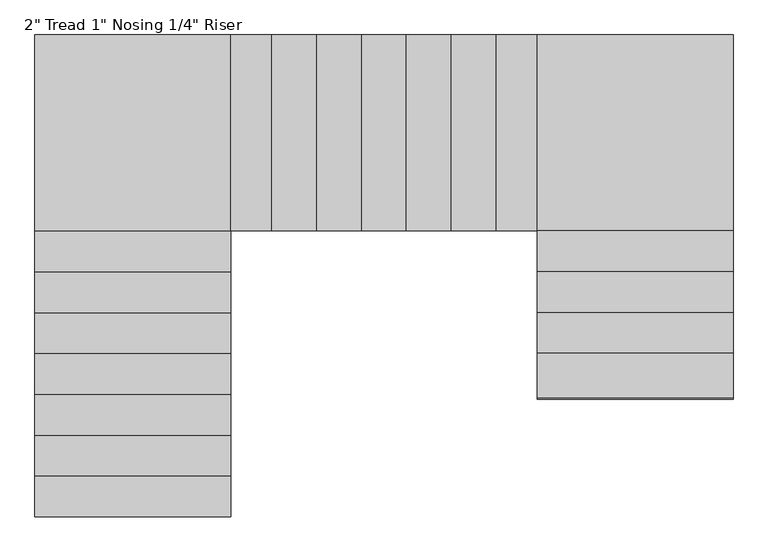
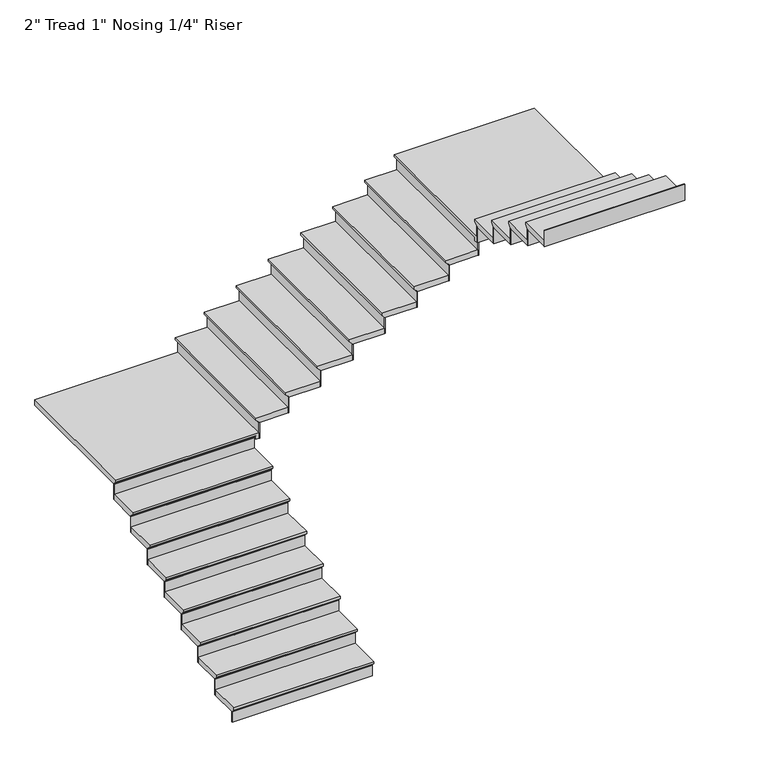
"""IFC4 building model written with IfcOpenShell, lengths in millimetres: stair flight geometry."""

from ifc_helpers import new_model, si_unit, origin, place, context, project, spatial, faceted_brep, source, transform, mapped, element, save


def stair_flight_02d0fc9c(model_context):
    return source(origin(), model_context, "Body", "Brep", [
        faceted_brep([(-39503.1146233, 12686.9618061, 6374.4928571), (-39503.1146233, 12686.9618061, 6393.5428571), (-40722.3146233, 12686.9618061, 6393.5428571), (-40722.3146233, 12686.9618061, 6374.4928571), (-39503.1146233, 12712.3618061, 6349.0928571), (-40722.3146233, 12712.3618061, 6349.0928571), (-39503.1146233, 12966.3618061, 6393.5428571), (-40722.3146233, 12966.3618061, 6393.5428571), (-40722.3146233, 12712.3618061, 6342.7428571), (-40722.3146233, 12966.3618061, 6342.7428571), (-39503.1146233, 12966.3618061, 6342.7428571), (-39503.1146233, 12712.3618061, 6342.7428571)], [[[0, 1, 2, 3]], [[4, 0, 3, 5]], [[2, 1, 6, 7]], [[8, 9, 10, 11]], [[2, 7, 9, 8, 5, 3]], [[8, 11, 4, 5]], [[6, 1, 0, 4, 11, 10]], [[7, 6, 10, 9]]]),
        faceted_brep([(-39503.1146233, 12712.3618061, 6342.7428571), (-39503.1146233, 12712.3618061, 6248.4), (-39503.1146233, 12718.7118061, 6248.4), (-39503.1146233, 12718.7118061, 6342.7428571), (-40722.3146233, 12712.3618061, 6342.7428571), (-40722.3146233, 12718.7118061, 6342.7428571), (-40722.3146233, 12718.7118061, 6248.4), (-40722.3146233, 12712.3618061, 6248.4)], [[[0, 1, 2, 3]], [[4, 5, 6, 7]], [[1, 0, 4, 7]], [[2, 1, 7, 6]], [[3, 2, 6, 5]], [[0, 3, 5, 4]]]),
        faceted_brep([(-39503.1146233, 12966.3618061, 6487.8857143), (-39503.1146233, 12966.3618061, 6342.7428571), (-39503.1146233, 12972.7118061, 6342.7428571), (-39503.1146233, 12972.7118061, 6487.8857143), (-40722.3146233, 12966.3618061, 6487.8857143), (-40722.3146233, 12972.7118061, 6487.8857143), (-40722.3146233, 12972.7118061, 6342.7428571), (-40722.3146233, 12966.3618061, 6342.7428571)], [[[0, 1, 2, 3]], [[4, 5, 6, 7]], [[1, 0, 4, 7]], [[2, 1, 7, 6]], [[3, 2, 6, 5]], [[0, 3, 5, 4]]]),
        faceted_brep([(-40722.3146233, 12940.9618061, 6538.6857143), (-39503.1146233, 12940.9618061, 6538.6857143), (-39503.1146233, 13220.3618061, 6538.6857143), (-40722.3146233, 13220.3618061, 6538.6857143), (-40722.3146233, 12966.3618061, 6487.8857143), (-40722.3146233, 13220.3618061, 6487.8857143), (-39503.1146233, 13220.3618061, 6487.8857143), (-39503.1146233, 12966.3618061, 6487.8857143), (-40722.3146233, 12966.3618061, 6494.2357143), (-40722.3146233, 12940.9618061, 6519.6357143), (-39503.1146233, 12966.3618061, 6494.2357143), (-39503.1146233, 12940.9618061, 6519.6357143)], [[[0, 1, 2, 3]], [[4, 5, 6, 7]], [[0, 3, 5, 4, 8, 9]], [[4, 7, 10, 8]], [[2, 1, 11, 10, 7, 6]], [[3, 2, 6, 5]], [[11, 1, 0, 9]], [[10, 11, 9, 8]]]),
        faceted_brep([(-39503.1146233, 13220.3618061, 6633.0285714), (-39503.1146233, 13220.3618061, 6487.8857143), (-39503.1146233, 13226.7118061, 6487.8857143), (-39503.1146233, 13226.7118061, 6633.0285714), (-40722.3146233, 13220.3618061, 6633.0285714), (-40722.3146233, 13226.7118061, 6633.0285714), (-40722.3146233, 13226.7118061, 6487.8857143), (-40722.3146233, 13220.3618061, 6487.8857143)], [[[0, 1, 2, 3]], [[4, 5, 6, 7]], [[1, 0, 4, 7]], [[2, 1, 7, 6]], [[3, 2, 6, 5]], [[0, 3, 5, 4]]]),
        faceted_brep([(-40722.3146233, 13194.9618061, 6683.8285714), (-39503.1146233, 13194.9618061, 6683.8285714), (-39503.1146233, 13474.3618061, 6683.8285714), (-40722.3146233, 13474.3618061, 6683.8285714), (-40722.3146233, 13220.3618061, 6633.0285714), (-40722.3146233, 13474.3618061, 6633.0285714), (-39503.1146233, 13474.3618061, 6633.0285714), (-39503.1146233, 13220.3618061, 6633.0285714), (-40722.3146233, 13220.3618061, 6639.3785714), (-40722.3146233, 13194.9618061, 6664.7785714), (-39503.1146233, 13220.3618061, 6639.3785714), (-39503.1146233, 13194.9618061, 6664.7785714)], [[[0, 1, 2, 3]], [[4, 5, 6, 7]], [[0, 3, 5, 4, 8, 9]], [[4, 7, 10, 8]], [[2, 1, 11, 10, 7, 6]], [[3, 2, 6, 5]], [[11, 1, 0, 9]], [[10, 11, 9, 8]]]),
        faceted_brep([(-39503.1146233, 13474.3618061, 6778.1714286), (-39503.1146233, 13474.3618061, 6633.0285714), (-39503.1146233, 13480.7118061, 6633.0285714), (-39503.1146233, 13480.7118061, 6778.1714286), (-40722.3146233, 13474.3618061, 6778.1714286), (-40722.3146233, 13480.7118061, 6778.1714286), (-40722.3146233, 13480.7118061, 6633.0285714), (-40722.3146233, 13474.3618061, 6633.0285714)], [[[0, 1, 2, 3]], [[4, 5, 6, 7]], [[1, 0, 4, 7]], [[2, 1, 7, 6]], [[3, 2, 6, 5]], [[0, 3, 5, 4]]]),
        faceted_brep([(-40722.3146233, 13448.9618061, 6828.9714286), (-39503.1146233, 13448.9618061, 6828.9714286), (-39503.1146233, 13728.3618061, 6828.9714286), (-40722.3146233, 13728.3618061, 6828.9714286), (-40722.3146233, 13474.3618061, 6778.1714286), (-40722.3146233, 13728.3618061, 6778.1714286), (-39503.1146233, 13728.3618061, 6778.1714286), (-39503.1146233, 13474.3618061, 6778.1714286), (-40722.3146233, 13474.3618061, 6784.5214286), (-40722.3146233, 13448.9618061, 6809.9214286), (-39503.1146233, 13474.3618061, 6784.5214286), (-39503.1146233, 13448.9618061, 6809.9214286)], [[[0, 1, 2, 3]], [[4, 5, 6, 7]], [[0, 3, 5, 4, 8, 9]], [[4, 7, 10, 8]], [[2, 1, 11, 10, 7, 6]], [[3, 2, 6, 5]], [[11, 1, 0, 9]], [[10, 11, 9, 8]]]),
        faceted_brep([(-39503.1146233, 13728.3618061, 6923.3142857), (-39503.1146233, 13728.3618061, 6778.1714286), (-39503.1146233, 13734.7118061, 6778.1714286), (-39503.1146233, 13734.7118061, 6923.3142857), (-40722.3146233, 13728.3618061, 6923.3142857), (-40722.3146233, 13734.7118061, 6923.3142857), (-40722.3146233, 13734.7118061, 6778.1714286), (-40722.3146233, 13728.3618061, 6778.1714286)], [[[0, 1, 2, 3]], [[4, 5, 6, 7]], [[1, 0, 4, 7]], [[2, 1, 7, 6]], [[3, 2, 6, 5]], [[0, 3, 5, 4]]]),
        faceted_brep([(-40722.3146233, 13702.9618061, 6974.1142857), (-39503.1146233, 13702.9618061, 6974.1142857), (-39503.1146233, 13982.3618061, 6974.1142857), (-40722.3146233, 13982.3618061, 6974.1142857), (-40722.3146233, 13728.3618061, 6923.3142857), (-40722.3146233, 13982.3618061, 6923.3142857), (-39503.1146233, 13982.3618061, 6923.3142857), (-39503.1146233, 13728.3618061, 6923.3142857), (-40722.3146233, 13728.3618061, 6929.6642857), (-40722.3146233, 13702.9618061, 6955.0642857), (-39503.1146233, 13728.3618061, 6929.6642857), (-39503.1146233, 13702.9618061, 6955.0642857)], [[[0, 1, 2, 3]], [[4, 5, 6, 7]], [[0, 3, 5, 4, 8, 9]], [[4, 7, 10, 8]], [[2, 1, 11, 10, 7, 6]], [[3, 2, 6, 5]], [[11, 1, 0, 9]], [[10, 11, 9, 8]]]),
        faceted_brep([(-39503.1146233, 13982.3618061, 7068.4571429), (-39503.1146233, 13982.3618061, 6923.3142857), (-39503.1146233, 13988.7118061, 6923.3142857), (-39503.1146233, 13988.7118061, 7068.4571429), (-40722.3146233, 13982.3618061, 7068.4571429), (-40722.3146233, 13988.7118061, 7068.4571429), (-40722.3146233, 13988.7118061, 6923.3142857), (-40722.3146233, 13982.3618061, 6923.3142857)], [[[0, 1, 2, 3]], [[4, 5, 6, 7]], [[1, 0, 4, 7]], [[2, 1, 7, 6]], [[3, 2, 6, 5]], [[0, 3, 5, 4]]]),
        faceted_brep([(-40722.3146233, 13956.9618061, 7119.2571429), (-39503.1146233, 13956.9618061, 7119.2571429), (-39503.1146233, 14236.3618061, 7119.2571429), (-40722.3146233, 14236.3618061, 7119.2571429), (-40722.3146233, 13982.3618061, 7068.4571429), (-40722.3146233, 14236.3618061, 7068.4571429), (-39503.1146233, 14236.3618061, 7068.4571429), (-39503.1146233, 13982.3618061, 7068.4571429), (-40722.3146233, 13982.3618061, 7074.8071429), (-40722.3146233, 13956.9618061, 7100.2071429), (-39503.1146233, 13982.3618061, 7074.8071429), (-39503.1146233, 13956.9618061, 7100.2071429)], [[[0, 1, 2, 3]], [[4, 5, 6, 7]], [[0, 3, 5, 4, 8, 9]], [[4, 7, 10, 8]], [[2, 1, 11, 10, 7, 6]], [[3, 2, 6, 5]], [[11, 1, 0, 9]], [[10, 11, 9, 8]]]),
        faceted_brep([(-39503.1146233, 14236.3618061, 7213.6), (-39503.1146233, 14236.3618061, 7068.4571429), (-39503.1146233, 14242.7118061, 7068.4571429), (-39503.1146233, 14242.7118061, 7213.6), (-40722.3146233, 14236.3618061, 7213.6), (-40722.3146233, 14242.7118061, 7213.6), (-40722.3146233, 14242.7118061, 7068.4571429), (-40722.3146233, 14236.3618061, 7068.4571429)], [[[0, 1, 2, 3]], [[4, 5, 6, 7]], [[1, 0, 4, 7]], [[2, 1, 7, 6]], [[3, 2, 6, 5]], [[0, 3, 5, 4]]]),
        faceted_brep([(-40722.3146233, 14210.9618061, 7264.4), (-39503.1146233, 14210.9618061, 7264.4), (-39503.1146233, 14490.3618061, 7264.4), (-40722.3146233, 14490.3618061, 7264.4), (-40722.3146233, 14236.3618061, 7213.6), (-40722.3146233, 14490.3618061, 7213.6), (-39503.1146233, 14490.3618061, 7213.6), (-39503.1146233, 14236.3618061, 7213.6), (-40722.3146233, 14236.3618061, 7219.95), (-40722.3146233, 14210.9618061, 7245.35), (-39503.1146233, 14236.3618061, 7219.95), (-39503.1146233, 14210.9618061, 7245.35)], [[[0, 1, 2, 3]], [[4, 5, 6, 7]], [[0, 3, 5, 4, 8, 9]], [[4, 7, 10, 8]], [[2, 1, 11, 10, 7, 6]], [[3, 2, 6, 5]], [[11, 1, 0, 9]], [[10, 11, 9, 8]]]),
        faceted_brep([(-39503.1146233, 14490.3618061, 7358.7428571), (-39503.1146233, 14490.3618061, 7213.6), (-39503.1146233, 14496.7118061, 7213.6), (-39503.1146233, 14496.7118061, 7358.7428571), (-40722.3146233, 14490.3618061, 7358.7428571), (-40722.3146233, 14496.7118061, 7358.7428571), (-40722.3146233, 14496.7118061, 7213.6), (-40722.3146233, 14490.3618061, 7213.6)], [[[0, 1, 2, 3]], [[4, 5, 6, 7]], [[1, 0, 4, 7]], [[2, 1, 7, 6]], [[3, 2, 6, 5]], [[0, 3, 5, 4]]]),
        faceted_brep([(-39477.7146233, 15684.1618061, 7409.5428571), (-40722.3146233, 15684.1618061, 7409.5428571), (-40722.3146233, 14464.9618061, 7409.5428571), (-39477.7146233, 14464.9618061, 7409.5428571), (-40722.3146233, 15684.1618061, 7358.7428571), (-39477.7146233, 15684.1618061, 7358.7428571), (-39477.7146233, 14464.9618061, 7358.7428571), (-39503.1146233, 14464.9618061, 7358.7428571), (-39503.1146233, 14490.3618061, 7358.7428571), (-40722.3146233, 14490.3618061, 7358.7428571), (-40722.3146233, 14490.3618061, 7365.0928571), (-40722.3146233, 14464.9618061, 7390.4928571), (-39503.1146233, 14490.3618061, 7365.0928571), (-39503.1146233, 14464.9618061, 7390.4928571)], [[[0, 1, 2, 3]], [[4, 5, 6, 7, 8, 9]], [[1, 0, 5, 4]], [[2, 1, 4, 9, 10, 11]], [[9, 8, 12, 10]], [[8, 7, 13, 12]], [[3, 2, 11, 13, 7, 6]], [[0, 3, 6, 5]], [[11, 10, 12, 13]]]),
        faceted_brep([(-39477.7146233, 14464.9618061, 7503.8857143), (-39477.7146233, 14464.9618061, 7358.7428571), (-39471.3646233, 14464.9618061, 7358.7428571), (-39471.3646233, 14464.9618061, 7503.8857143), (-39477.7146233, 15684.1618061, 7503.8857143), (-39471.3646233, 15684.1618061, 7503.8857143), (-39471.3646233, 15684.1618061, 7358.7428571), (-39477.7146233, 15684.1618061, 7358.7428571)], [[[0, 1, 2, 3]], [[4, 5, 6, 7]], [[1, 0, 4, 7]], [[2, 1, 7, 6]], [[3, 2, 6, 5]], [[0, 3, 5, 4]]]),
        faceted_brep([(-39503.1146233, 15684.1618061, 7554.6857143), (-39503.1146233, 14464.9618061, 7554.6857143), (-39223.7146233, 14464.9618061, 7554.6857143), (-39223.7146233, 15684.1618061, 7554.6857143), (-39477.7146233, 15684.1618061, 7503.8857143), (-39223.7146233, 15684.1618061, 7503.8857143), (-39223.7146233, 14464.9618061, 7503.8857143), (-39477.7146233, 14464.9618061, 7503.8857143), (-39477.7146233, 15684.1618061, 7510.2357143), (-39503.1146233, 15684.1618061, 7535.6357143), (-39477.7146233, 14464.9618061, 7510.2357143), (-39503.1146233, 14464.9618061, 7535.6357143)], [[[0, 1, 2, 3]], [[4, 5, 6, 7]], [[0, 3, 5, 4, 8, 9]], [[4, 7, 10, 8]], [[2, 1, 11, 10, 7, 6]], [[3, 2, 6, 5]], [[11, 1, 0, 9]], [[10, 11, 9, 8]]]),
        faceted_brep([(-39223.7146233, 14464.9618061, 7649.0285714), (-39223.7146233, 14464.9618061, 7503.8857143), (-39217.3646233, 14464.9618061, 7503.8857143), (-39217.3646233, 14464.9618061, 7649.0285714), (-39223.7146233, 15684.1618061, 7649.0285714), (-39217.3646233, 15684.1618061, 7649.0285714), (-39217.3646233, 15684.1618061, 7503.8857143), (-39223.7146233, 15684.1618061, 7503.8857143)], [[[0, 1, 2, 3]], [[4, 5, 6, 7]], [[1, 0, 4, 7]], [[2, 1, 7, 6]], [[3, 2, 6, 5]], [[0, 3, 5, 4]]]),
        faceted_brep([(-39249.1146233, 15684.1618061, 7699.8285714), (-39249.1146233, 14464.9618061, 7699.8285714), (-38944.3146233, 14464.9618061, 7699.8285714), (-38944.3146233, 15684.1618061, 7699.8285714), (-39223.7146233, 15684.1618061, 7649.0285714), (-38944.3146233, 15684.1618061, 7649.0285714), (-38944.3146233, 14464.9618061, 7649.0285714), (-39223.7146233, 14464.9618061, 7649.0285714), (-39223.7146233, 15684.1618061, 7655.3785714), (-39249.1146233, 15684.1618061, 7680.7785714), (-39223.7146233, 14464.9618061, 7655.3785714), (-39249.1146233, 14464.9618061, 7680.7785714)], [[[0, 1, 2, 3]], [[4, 5, 6, 7]], [[0, 3, 5, 4, 8, 9]], [[4, 7, 10, 8]], [[2, 1, 11, 10, 7, 6]], [[3, 2, 6, 5]], [[11, 1, 0, 9]], [[10, 11, 9, 8]]]),
        faceted_brep([(-38944.3146233, 14464.9618061, 7794.1714286), (-38944.3146233, 14464.9618061, 7649.0285714), (-38937.9646233, 14464.9618061, 7649.0285714), (-38937.9646233, 14464.9618061, 7794.1714286), (-38944.3146233, 15684.1618061, 7794.1714286), (-38937.9646233, 15684.1618061, 7794.1714286), (-38937.9646233, 15684.1618061, 7649.0285714), (-38944.3146233, 15684.1618061, 7649.0285714)], [[[0, 1, 2, 3]], [[4, 5, 6, 7]], [[1, 0, 4, 7]], [[2, 1, 7, 6]], [[3, 2, 6, 5]], [[0, 3, 5, 4]]]),
        faceted_brep([(-38969.7146233, 15684.1618061, 7844.9714286), (-38969.7146233, 14464.9618061, 7844.9714286), (-38664.9146233, 14464.9618061, 7844.9714286), (-38664.9146233, 15684.1618061, 7844.9714286), (-38944.3146233, 15684.1618061, 7794.1714286), (-38664.9146233, 15684.1618061, 7794.1714286), (-38664.9146233, 14464.9618061, 7794.1714286), (-38944.3146233, 14464.9618061, 7794.1714286), (-38944.3146233, 15684.1618061, 7800.5214286), (-38969.7146233, 15684.1618061, 7825.9214286), (-38944.3146233, 14464.9618061, 7800.5214286), (-38969.7146233, 14464.9618061, 7825.9214286)], [[[0, 1, 2, 3]], [[4, 5, 6, 7]], [[0, 3, 5, 4, 8, 9]], [[4, 7, 10, 8]], [[2, 1, 11, 10, 7, 6]], [[3, 2, 6, 5]], [[11, 1, 0, 9]], [[10, 11, 9, 8]]]),
        faceted_brep([(-38664.9146233, 14464.9618061, 7939.3142857), (-38664.9146233, 14464.9618061, 7794.1714286), (-38658.5646233, 14464.9618061, 7794.1714286), (-38658.5646233, 14464.9618061, 7939.3142857), (-38664.9146233, 15684.1618061, 7939.3142857), (-38658.5646233, 15684.1618061, 7939.3142857), (-38658.5646233, 15684.1618061, 7794.1714286), (-38664.9146233, 15684.1618061, 7794.1714286)], [[[0, 1, 2, 3]], [[4, 5, 6, 7]], [[1, 0, 4, 7]], [[2, 1, 7, 6]], [[3, 2, 6, 5]], [[0, 3, 5, 4]]]),
        faceted_brep([(-38690.3146233, 15684.1618061, 7990.1142857), (-38690.3146233, 14464.9618061, 7990.1142857), (-38385.5146233, 14464.9618061, 7990.1142857), (-38385.5146233, 15684.1618061, 7990.1142857), (-38664.9146233, 15684.1618061, 7939.3142857), (-38385.5146233, 15684.1618061, 7939.3142857), (-38385.5146233, 14464.9618061, 7939.3142857), (-38664.9146233, 14464.9618061, 7939.3142857), (-38664.9146233, 15684.1618061, 7945.6642857), (-38690.3146233, 15684.1618061, 7971.0642857), (-38664.9146233, 14464.9618061, 7945.6642857), (-38690.3146233, 14464.9618061, 7971.0642857)], [[[0, 1, 2, 3]], [[4, 5, 6, 7]], [[0, 3, 5, 4, 8, 9]], [[4, 7, 10, 8]], [[2, 1, 11, 10, 7, 6]], [[3, 2, 6, 5]], [[11, 1, 0, 9]], [[10, 11, 9, 8]]]),
        faceted_brep([(-38385.5146233, 14464.9618061, 8084.4571429), (-38385.5146233, 14464.9618061, 7939.3142857), (-38379.1646233, 14464.9618061, 7939.3142857), (-38379.1646233, 14464.9618061, 8084.4571429), (-38385.5146233, 15684.1618061, 8084.4571429), (-38379.1646233, 15684.1618061, 8084.4571429), (-38379.1646233, 15684.1618061, 7939.3142857), (-38385.5146233, 15684.1618061, 7939.3142857)], [[[0, 1, 2, 3]], [[4, 5, 6, 7]], [[1, 0, 4, 7]], [[2, 1, 7, 6]], [[3, 2, 6, 5]], [[0, 3, 5, 4]]]),
        faceted_brep([(-38410.9146233, 15684.1618061, 8135.2571429), (-38410.9146233, 14464.9618061, 8135.2571429), (-38106.1146233, 14464.9618061, 8135.2571429), (-38106.1146233, 15684.1618061, 8135.2571429), (-38385.5146233, 15684.1618061, 8084.4571429), (-38106.1146233, 15684.1618061, 8084.4571429), (-38106.1146233, 14464.9618061, 8084.4571429), (-38385.5146233, 14464.9618061, 8084.4571429), (-38385.5146233, 15684.1618061, 8090.8071429), (-38410.9146233, 15684.1618061, 8116.2071429), (-38385.5146233, 14464.9618061, 8090.8071429), (-38410.9146233, 14464.9618061, 8116.2071429)], [[[0, 1, 2, 3]], [[4, 5, 6, 7]], [[0, 3, 5, 4, 8, 9]], [[4, 7, 10, 8]], [[2, 1, 11, 10, 7, 6]], [[3, 2, 6, 5]], [[11, 1, 0, 9]], [[10, 11, 9, 8]]]),
        faceted_brep([(-38106.1146233, 14464.9618061, 8229.6), (-38106.1146233, 14464.9618061, 8084.4571429), (-38099.7646233, 14464.9618061, 8084.4571429), (-38099.7646233, 14464.9618061, 8229.6), (-38106.1146233, 15684.1618061, 8229.6), (-38099.7646233, 15684.1618061, 8229.6), (-38099.7646233, 15684.1618061, 8084.4571429), (-38106.1146233, 15684.1618061, 8084.4571429)], [[[0, 1, 2, 3]], [[4, 5, 6, 7]], [[1, 0, 4, 7]], [[2, 1, 7, 6]], [[3, 2, 6, 5]], [[0, 3, 5, 4]]]),
        faceted_brep([(-38131.5146233, 15684.1618061, 8280.4), (-38131.5146233, 14464.9618061, 8280.4), (-37826.7146233, 14464.9618061, 8280.4), (-37826.7146233, 15684.1618061, 8280.4), (-38106.1146233, 15684.1618061, 8229.6), (-37826.7146233, 15684.1618061, 8229.6), (-37826.7146233, 14464.9618061, 8229.6), (-38106.1146233, 14464.9618061, 8229.6), (-38106.1146233, 15684.1618061, 8235.95), (-38131.5146233, 15684.1618061, 8261.35), (-38106.1146233, 14464.9618061, 8235.95), (-38131.5146233, 14464.9618061, 8261.35)], [[[0, 1, 2, 3]], [[4, 5, 6, 7]], [[0, 3, 5, 4, 8, 9]], [[4, 7, 10, 8]], [[2, 1, 11, 10, 7, 6]], [[3, 2, 6, 5]], [[11, 1, 0, 9]], [[10, 11, 9, 8]]]),
        faceted_brep([(-37826.7146233, 14464.9618061, 8374.7428571), (-37826.7146233, 14464.9618061, 8229.6), (-37820.3646233, 14464.9618061, 8229.6), (-37820.3646233, 14464.9618061, 8374.7428571), (-37826.7146233, 15684.1618061, 8374.7428571), (-37820.3646233, 15684.1618061, 8374.7428571), (-37820.3646233, 15684.1618061, 8229.6), (-37826.7146233, 15684.1618061, 8229.6)], [[[0, 1, 2, 3]], [[4, 5, 6, 7]], [[1, 0, 4, 7]], [[2, 1, 7, 6]], [[3, 2, 6, 5]], [[0, 3, 5, 4]]]),
        faceted_brep([(-37852.1146233, 15684.1618061, 8425.5428571), (-37852.1146233, 14464.9618061, 8425.5428571), (-37572.7146233, 14464.9618061, 8425.5428571), (-37572.7146233, 15684.1618061, 8425.5428571), (-37826.7146233, 15684.1618061, 8374.7428571), (-37572.7146233, 15684.1618061, 8374.7428571), (-37572.7146233, 14464.9618061, 8374.7428571), (-37826.7146233, 14464.9618061, 8374.7428571), (-37826.7146233, 15684.1618061, 8381.0928571), (-37852.1146233, 15684.1618061, 8406.4928571), (-37826.7146233, 14464.9618061, 8381.0928571), (-37852.1146233, 14464.9618061, 8406.4928571)], [[[0, 1, 2, 3]], [[4, 5, 6, 7]], [[0, 3, 5, 4, 8, 9]], [[4, 7, 10, 8]], [[2, 1, 11, 10, 7, 6]], [[3, 2, 6, 5]], [[11, 1, 0, 9]], [[10, 11, 9, 8]]]),
        faceted_brep([(-37572.7146233, 14464.9618061, 8519.8857143), (-37572.7146233, 14464.9618061, 8374.7428571), (-37566.3646233, 14464.9618061, 8374.7428571), (-37566.3646233, 14464.9618061, 8519.8857143), (-37572.7146233, 15684.1618061, 8519.8857143), (-37566.3646233, 15684.1618061, 8519.8857143), (-37566.3646233, 15684.1618061, 8374.7428571), (-37572.7146233, 15684.1618061, 8374.7428571)], [[[0, 1, 2, 3]], [[4, 5, 6, 7]], [[1, 0, 4, 7]], [[2, 1, 7, 6]], [[3, 2, 6, 5]], [[0, 3, 5, 4]]]),
        faceted_brep([(-36378.9146233, 14439.5618061, 8570.6857143), (-36378.9146233, 15684.1618061, 8570.6857143), (-37598.1146233, 15684.1618061, 8570.6857143), (-37598.1146233, 14439.5618061, 8570.6857143), (-36378.9146233, 15684.1618061, 8519.8857143), (-36378.9146233, 14439.5618061, 8519.8857143), (-37598.1146233, 14439.5618061, 8519.8857143), (-37598.1146233, 14464.9618061, 8519.8857143), (-37572.7146233, 14464.9618061, 8519.8857143), (-37572.7146233, 15684.1618061, 8519.8857143), (-37572.7146233, 15684.1618061, 8526.2357143), (-37598.1146233, 15684.1618061, 8551.6357143), (-37572.7146233, 14464.9618061, 8526.2357143), (-37598.1146233, 14464.9618061, 8551.6357143)], [[[0, 1, 2, 3]], [[4, 5, 6, 7, 8, 9]], [[1, 0, 5, 4]], [[2, 1, 4, 9, 10, 11]], [[9, 8, 12, 10]], [[8, 7, 13, 12]], [[3, 2, 11, 13, 7, 6]], [[0, 3, 6, 5]], [[11, 10, 12, 13]]]),
        faceted_brep([(-37598.1146233, 14439.5618061, 8665.0285714), (-37598.1146233, 14439.5618061, 8519.8857143), (-37598.1146233, 14433.2118061, 8519.8857143), (-37598.1146233, 14433.2118061, 8665.0285714), (-36378.9146233, 14439.5618061, 8665.0285714), (-36378.9146233, 14433.2118061, 8665.0285714), (-36378.9146233, 14433.2118061, 8519.8857143), (-36378.9146233, 14439.5618061, 8519.8857143)], [[[0, 1, 2, 3]], [[4, 5, 6, 7]], [[1, 0, 4, 7]], [[2, 1, 7, 6]], [[3, 2, 6, 5]], [[0, 3, 5, 4]]]),
        faceted_brep([(-36378.9146233, 14464.9618061, 8715.8285714), (-37598.1146233, 14464.9618061, 8715.8285714), (-37598.1146233, 14185.5618061, 8715.8285714), (-36378.9146233, 14185.5618061, 8715.8285714), (-36378.9146233, 14439.5618061, 8665.0285714), (-36378.9146233, 14185.5618061, 8665.0285714), (-37598.1146233, 14185.5618061, 8665.0285714), (-37598.1146233, 14439.5618061, 8665.0285714), (-36378.9146233, 14439.5618061, 8671.3785714), (-36378.9146233, 14464.9618061, 8696.7785714), (-37598.1146233, 14439.5618061, 8671.3785714), (-37598.1146233, 14464.9618061, 8696.7785714)], [[[0, 1, 2, 3]], [[4, 5, 6, 7]], [[0, 3, 5, 4, 8, 9]], [[4, 7, 10, 8]], [[2, 1, 11, 10, 7, 6]], [[3, 2, 6, 5]], [[11, 1, 0, 9]], [[10, 11, 9, 8]]]),
        faceted_brep([(-37598.1146233, 14185.5618061, 8810.1714286), (-37598.1146233, 14185.5618061, 8665.0285714), (-37598.1146233, 14179.2118061, 8665.0285714), (-37598.1146233, 14179.2118061, 8810.1714286), (-36378.9146233, 14185.5618061, 8810.1714286), (-36378.9146233, 14179.2118061, 8810.1714286), (-36378.9146233, 14179.2118061, 8665.0285714), (-36378.9146233, 14185.5618061, 8665.0285714)], [[[0, 1, 2, 3]], [[4, 5, 6, 7]], [[1, 0, 4, 7]], [[2, 1, 7, 6]], [[3, 2, 6, 5]], [[0, 3, 5, 4]]]),
        faceted_brep([(-36378.9146233, 14210.9618061, 8860.9714286), (-37598.1146233, 14210.9618061, 8860.9714286), (-37598.1146233, 13931.5618061, 8860.9714286), (-36378.9146233, 13931.5618061, 8860.9714286), (-36378.9146233, 14185.5618061, 8810.1714286), (-36378.9146233, 13931.5618061, 8810.1714286), (-37598.1146233, 13931.5618061, 8810.1714286), (-37598.1146233, 14185.5618061, 8810.1714286), (-36378.9146233, 14185.5618061, 8816.5214286), (-36378.9146233, 14210.9618061, 8841.9214286), (-37598.1146233, 14185.5618061, 8816.5214286), (-37598.1146233, 14210.9618061, 8841.9214286)], [[[0, 1, 2, 3]], [[4, 5, 6, 7]], [[0, 3, 5, 4, 8, 9]], [[4, 7, 10, 8]], [[2, 1, 11, 10, 7, 6]], [[3, 2, 6, 5]], [[11, 1, 0, 9]], [[10, 11, 9, 8]]]),
        faceted_brep([(-37598.1146233, 13931.5618061, 8955.3142857), (-37598.1146233, 13931.5618061, 8810.1714286), (-37598.1146233, 13925.2118061, 8810.1714286), (-37598.1146233, 13925.2118061, 8955.3142857), (-36378.9146233, 13931.5618061, 8955.3142857), (-36378.9146233, 13925.2118061, 8955.3142857), (-36378.9146233, 13925.2118061, 8810.1714286), (-36378.9146233, 13931.5618061, 8810.1714286)], [[[0, 1, 2, 3]], [[4, 5, 6, 7]], [[1, 0, 4, 7]], [[2, 1, 7, 6]], [[3, 2, 6, 5]], [[0, 3, 5, 4]]]),
        faceted_brep([(-36378.9146233, 13956.9618061, 9006.1142857), (-37598.1146233, 13956.9618061, 9006.1142857), (-37598.1146233, 13677.5618061, 9006.1142857), (-36378.9146233, 13677.5618061, 9006.1142857), (-36378.9146233, 13931.5618061, 8955.3142857), (-36378.9146233, 13677.5618061, 8955.3142857), (-37598.1146233, 13677.5618061, 8955.3142857), (-37598.1146233, 13931.5618061, 8955.3142857), (-36378.9146233, 13931.5618061, 8961.6642857), (-36378.9146233, 13956.9618061, 8987.0642857), (-37598.1146233, 13931.5618061, 8961.6642857), (-37598.1146233, 13956.9618061, 8987.0642857)], [[[0, 1, 2, 3]], [[4, 5, 6, 7]], [[0, 3, 5, 4, 8, 9]], [[4, 7, 10, 8]], [[2, 1, 11, 10, 7, 6]], [[3, 2, 6, 5]], [[11, 1, 0, 9]], [[10, 11, 9, 8]]]),
        faceted_brep([(-37598.1146233, 13677.5618061, 9100.4571429), (-37598.1146233, 13677.5618061, 8955.3142857), (-37598.1146233, 13671.2118061, 8955.3142857), (-37598.1146233, 13671.2118061, 9100.4571429), (-36378.9146233, 13677.5618061, 9100.4571429), (-36378.9146233, 13671.2118061, 9100.4571429), (-36378.9146233, 13671.2118061, 8955.3142857), (-36378.9146233, 13677.5618061, 8955.3142857)], [[[0, 1, 2, 3]], [[4, 5, 6, 7]], [[1, 0, 4, 7]], [[2, 1, 7, 6]], [[3, 2, 6, 5]], [[0, 3, 5, 4]]]),
        faceted_brep([(-37598.1146233, 13423.5618061, 9245.6), (-37598.1146233, 13423.5618061, 9100.4571429), (-37598.1146233, 13417.2118061, 9100.4571429), (-37598.1146233, 13417.2118061, 9245.6), (-36378.9146233, 13423.5618061, 9245.6), (-36378.9146233, 13417.2118061, 9245.6), (-36378.9146233, 13417.2118061, 9100.4571429), (-36378.9146233, 13423.5618061, 9100.4571429)], [[[0, 1, 2, 3]], [[4, 5, 6, 7]], [[1, 0, 4, 7]], [[2, 1, 7, 6]], [[3, 2, 6, 5]], [[0, 3, 5, 4]]]),
        faceted_brep([(-36378.9146233, 13702.9618061, 9151.2571429), (-37598.1146233, 13702.9618061, 9151.2571429), (-37598.1146233, 13423.5618061, 9151.2571429), (-36378.9146233, 13423.5618061, 9151.2571429), (-36378.9146233, 13677.5618061, 9100.4571429), (-36378.9146233, 13423.5618061, 9100.4571429), (-37598.1146233, 13423.5618061, 9100.4571429), (-37598.1146233, 13677.5618061, 9100.4571429), (-36378.9146233, 13677.5618061, 9106.8071429), (-36378.9146233, 13702.9618061, 9132.2071429), (-37598.1146233, 13677.5618061, 9106.8071429), (-37598.1146233, 13702.9618061, 9132.2071429)], [[[0, 1, 2, 3]], [[4, 5, 6, 7]], [[0, 3, 5, 4, 8, 9]], [[4, 7, 10, 8]], [[2, 1, 11, 10, 7, 6]], [[3, 2, 6, 5]], [[11, 1, 0, 9]], [[10, 11, 9, 8]]]),
    ])


if __name__ == "__main__":
    model = new_model("IFC4")
    model_context = context("Model", 3, world=origin())
    ifc_project = project(units=[si_unit("LENGTHUNIT", "METRE", prefix="MILLI")], contexts=[model_context])
    site = spatial("IfcSite", under=ifc_project)
    building = spatial("IfcBuilding", under=site)
    placement = place(None, origin())
    stair_flight_shape = stair_flight_02d0fc9c(model_context)
    element("IfcStairFlight", 1, ObjectType="2\" Tread 1\" Nosing 1/4\" Riser", at=placement, inside=building, context=model_context, shape_type="MappedRepresentation", body=[
        mapped(stair_flight_shape, transform((0.0, 0.0, 0.0), x_axis=(1.0, 0.0, 0.0), y_axis=(0.0, 1.0, 0.0), z_axis=(0.0, 0.0, 1.0))),
    ])
    save(model, "model.ifc")
